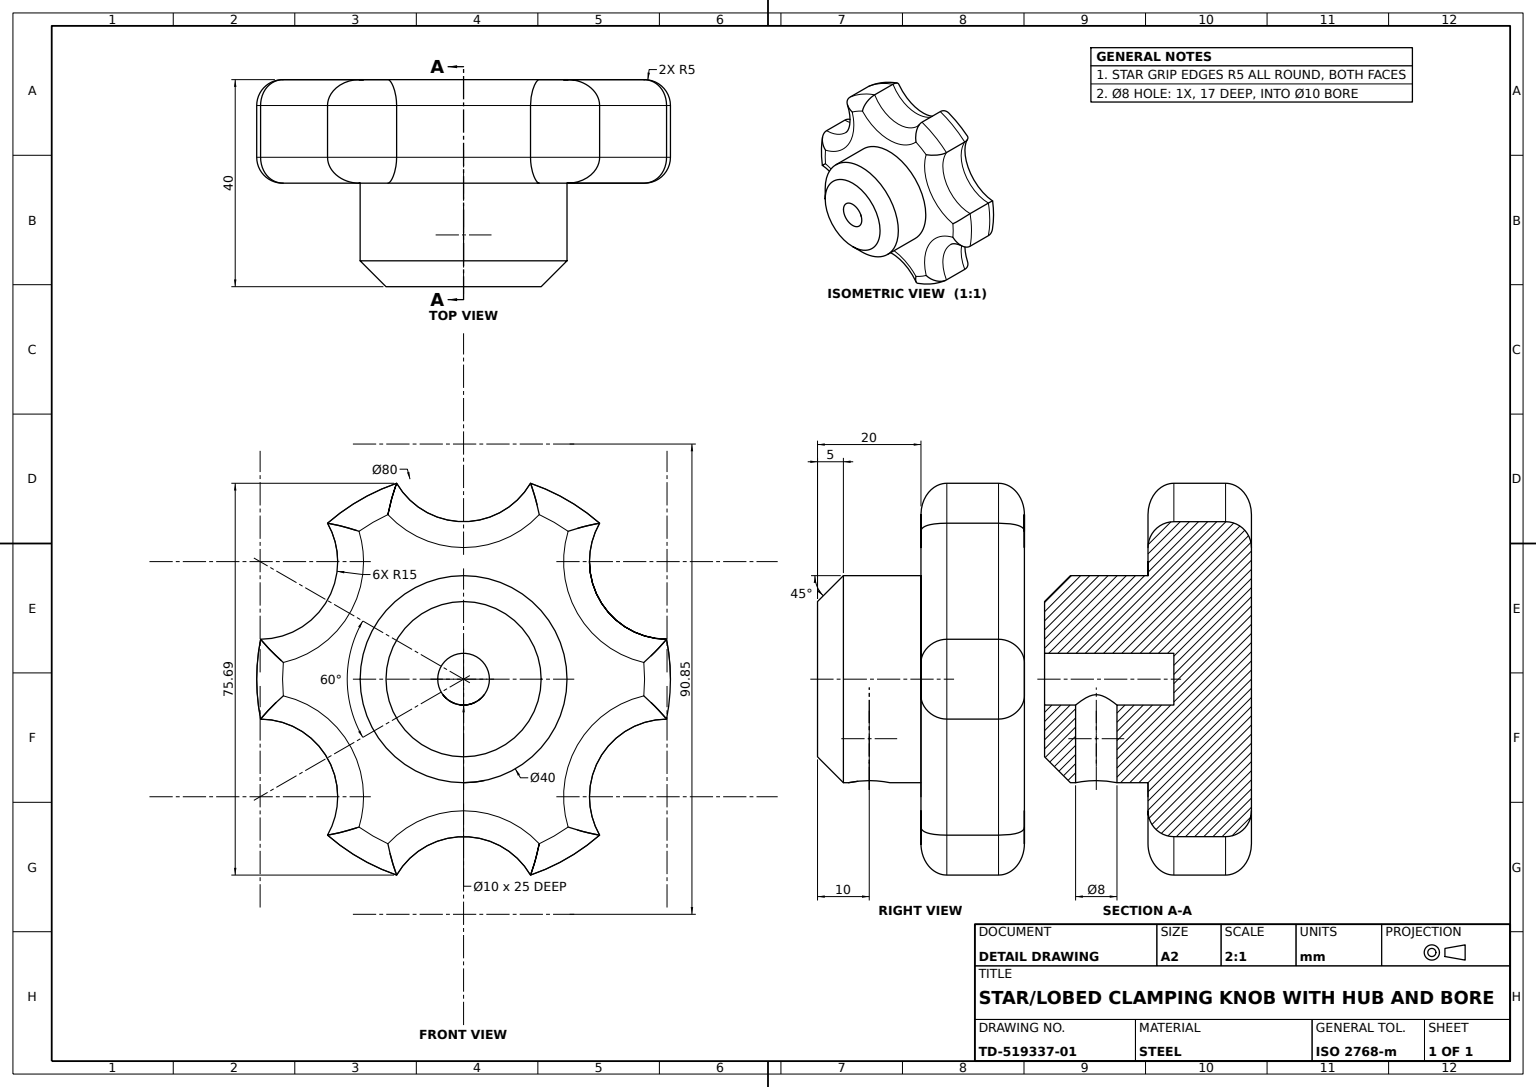
from build123d import *

# Parameters (mm, degrees)
STAR_GRIP_BODY_DEPTH    = 20
HUB_SKETCH_R            = 20
HUB_SKETCH_R_2          = 17.5
HUB_BOSS_40_DEPTH       = 20
BORE_SKETCH_R           = 5
AXIAL_BORE_10_DEPTH     = 25
SET_SCREW_HOLE_SKETCH_R = 4
SET_SCREW_HOLE_8_DEPTH  = 24
HUB_CHAMFER_5X45_SIZE   = 5
GRIP_EDGE_FILLET_R5_A_R = 5
GRIP_EDGE_FILLET_R5_B_R = 5


with BuildPart() as part:
    # Star Grip Profile Sketch → Star Grip Body (new body)
    with BuildSketch(Plane.XY):
        with BuildLine():
            ThreePointArc((-39.249340356, 7.71292951), (-40, 0), (-39.249340356, -7.71292951))
            ThreePointArc((-39.249340356, -7.71292951), (-26.349097745, -15.212658676), (-26.304263071, -30.134461075))
            ThreePointArc((-26.304263071, -30.134461075), (-20, -34.641016151), (-12.945077285, -37.847390585))
            ThreePointArc((-12.945077285, -37.847390585), (0, -30.425317352), (12.945077285, -37.847390585))
            ThreePointArc((12.945077285, -37.847390585), (20, -34.641016151), (26.304263071, -30.134461075))
            ThreePointArc((26.304263071, -30.134461075), (26.349097745, -15.212658676), (39.249340356, -7.71292951))
            ThreePointArc((39.249340356, -7.71292951), (40, 0), (39.249340356, 7.71292951))
            ThreePointArc((39.249340356, 7.71292951), (26.349097745, 15.212658676), (26.304263071, 30.134461075))
            ThreePointArc((26.304263071, 30.134461075), (20, 34.641016151), (12.945077285, 37.847390585))
            ThreePointArc((12.945077285, 37.847390585), (0, 30.425317352), (-12.945077285, 37.847390585))
            ThreePointArc((-12.945077285, 37.847390585), (-20, 34.641016151), (-26.304263071, 30.134461075))
            ThreePointArc((-26.304263071, 30.134461075), (-26.349097745, 15.212658676), (-39.249340356, 7.71292951))
        make_face()
    extrude(amount=STAR_GRIP_BODY_DEPTH)

    # Hub Sketch → Hub Boss Ø40 (add)
    # profile 1 of 2: a face of its own
    with BuildSketch(Plane.XY.offset(20)):
        Circle(HUB_SKETCH_R)
        Circle(HUB_SKETCH_R_2, mode=Mode.SUBTRACT)
    # profile 2 of 2: a face of its own
    with BuildSketch(Plane.XY.offset(20)):
        Circle(HUB_SKETCH_R_2)
    extrude(amount=HUB_BOSS_40_DEPTH)

    # Bore Sketch → Axial Bore Ø10 (cut)
    with BuildSketch(Plane.XY.offset(40)):
        Circle(BORE_SKETCH_R)
    extrude(amount=-AXIAL_BORE_10_DEPTH, mode=Mode.SUBTRACT)

    # Set Screw Hole Sketch → Set Screw Hole Ø8 (cut)
    with BuildSketch(Plane(origin=(0, 0, 0), x_dir=(1, 0, 0), z_dir=(0, 1, 0))):
        with Locations(Location((0, -30, 0), (0, 0, 270))):
            Circle(SET_SCREW_HOLE_SKETCH_R)
    extrude(amount=-SET_SCREW_HOLE_8_DEPTH, mode=Mode.SUBTRACT)

    # Hub Chamfer 5x45
    hub_chamfer_5x45_edges = [part.edges().sort_by_distance(p)[0] for p in [
        (-20, 0, 40),
    ]]
    chamfer(hub_chamfer_5x45_edges, length=HUB_CHAMFER_5X45_SIZE)

    # Grip Edge Fillet R5 A
    grip_edge_fillet_r5_a_edges = [part.edges().sort_by_distance(p)[0] for p in [
        (-20, 34.641016151, 20),
        (-26.349097745, 15.212658676, 20),
        (-40, 0, 20),
        (-26.349097745, -15.212658676, 20),
        (-20, -34.641016151, 20),
        (0, -30.425317352, 20),
        (20, -34.641016151, 20),
        (26.349097745, -15.212658676, 20),
        (40, 0, 20),
        (26.349097745, 15.212658676, 20),
        (20, 34.641016151, 20),
        (0, 30.425317352, 20),
    ]]
    fillet(grip_edge_fillet_r5_a_edges, radius=GRIP_EDGE_FILLET_R5_A_R)

    # Grip Edge Fillet R5 B
    grip_edge_fillet_r5_b_edges = [part.edges().sort_by_distance(p)[0] for p in [
        (26.349097745, 15.212658676, 0),
        (40, 0, 0),
        (26.349097745, -15.212658676, 0),
        (20, -34.641016151, 0),
        (0, -30.425317352, 0),
        (-20, -34.641016151, 0),
        (-26.349097745, -15.212658676, 0),
        (-40, 0, 0),
        (-26.349097745, 15.212658676, 0),
        (-20, 34.641016151, 0),
        (0, 30.425317352, 0),
        (20, 34.641016151, 0),
    ]]
    fillet(grip_edge_fillet_r5_b_edges, radius=GRIP_EDGE_FILLET_R5_B_R)


solid = part.part
